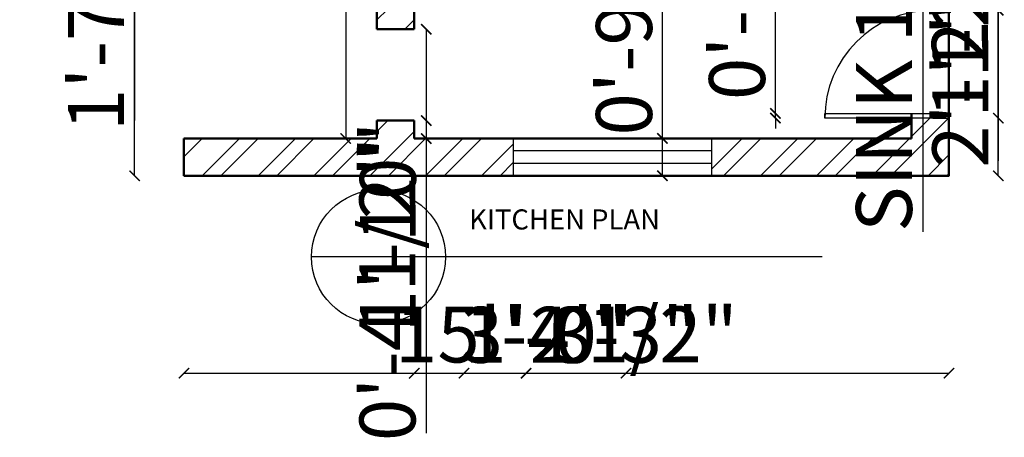
# Model space of a CAD drawing. Units: inches. Extents: x 1736 to 2023, y 1717 to 2014.
# Tile 1 of 3: x 1736 to 1974, y 1717 to 1818. Entities that reach past the tile are written whole.
import ezdxf

# ---------------------------------------------------------------- set-up
doc = ezdxf.new("R2010")
doc.units = ezdxf.units.IN
for name, color, linetype, lineweight in [('A-ANNO-DIMS', 2, 'Continuous', 18), ('A-ANNO-SYMB', 7, 'Continuous', 25), ('A-DOOR', 4, 'Continuous', 25), ('A-GLAZ', 4, 'Continuous', 25), ('A-WALL', 7, 'Continuous', 50), ('A-WALL-PATT', 8, 'Continuous', 13)]:
    doc.layers.add(name, color=color, linetype=linetype, lineweight=lineweight)
doc.styles.get("Standard").update_dxf_attribs({"font": 'arial.ttf'})
doc.dimstyles.new('ISO-25', dxfattribs={"dimtxt": 13.5, "dimasz": 2.5, "dimexe": 1.25, "dimexo": 0.625, "dimtad": 1, "dimdec": 0, "dimlunit": 4, "dimtxsty": 'Standard', "dimblk": 'ARCHTICK', "dimcen": 2.5, "dimse1": 1, "dimse2": 1, "dimclrd": 2, "dimclrt": 4, "dimadec": 0, "dimazin": 0, "dimtfac": 1, "dimtdec": 0, "dimtmove": 0, "dimatfit": 3, "dimfxl": 1, "dimarcsym": 0})

# ---------------------------------------------------------------- blocks, each defined once
blk = doc.blocks.new('*U4')
for p, q in [((0, 0), (0, -6)), ((40, 0), (40, -6))]:
    blk.add_line(p, q)
blk.add_lwpolyline([(0, 0), (0, 40), (1.75, 40), (1.75, 0)], close=True)
blk.add_arc((0, 0), 40, 0, 90)
blk = doc.blocks.new('_ArchTick')
at = {"color": 0, "linetype": 'ByBlock', "const_width": 0.15}
blk.add_lwpolyline([(-0.5, -0.5), (0.5, 0.5)], dxfattribs=at)
blk = doc.blocks.new('*D8')
at = {"layer": 'A-ANNO-DIMS', "color": 0, "lineweight": -2, "transparency": 16777216}
blk.add_line((1814.91, 1933.29), (1814.91, 1789.29), dxfattribs=at)
at = {"layer": 'Defpoints', "color": 0, "transparency": 16777216}
for p in [(1822.43, 1933.29), (1814.91, 1789.29), (1822.43, 1789.29)]:
    blk.add_point(p, dxfattribs=at)
at = {"layer": 'A-ANNO-DIMS', "color": 0, "lineweight": -2, "transparency": 16777216, "xscale": 2.5, "yscale": 2.5, "zscale": 2.5}
for p, rotation in [((1814.91, 1933.29), 90), ((1814.91, 1789.29), 270)]:
    blk.add_blockref('_ArchTick', p, dxfattribs=dict(at, rotation=rotation))
at = {"layer": 'A-ANNO-DIMS', "color": 0, "transparency": 16777216, "insert": (1807.51, 1861.29), "char_height": 13.5, "attachment_point": 5, "rotation": 90}
blk.add_mtext("12'", dxfattribs=at)
blk = doc.blocks.new('*D11')
at = {"layer": 'A-ANNO-DIMS', "color": 2, "lineweight": -2, "transparency": 16777216}
for p, q in [((1954.12, 1873.5), (1954.12, 1855.61)), ((1954.12, 1855.61), (1954.12, 1766.78))]:
    blk.add_line(p, q, dxfattribs=at)
at = {"layer": 'Defpoints', "color": 0, "transparency": 16777216}
for p in [(1951.43, 1873.5), (1951.43, 1855.61), (1954.12, 1855.61)]:
    blk.add_point(p, dxfattribs=at)
at = {"layer": 'A-ANNO-DIMS', "color": 2, "lineweight": -2, "transparency": 16777216, "xscale": 2.5, "yscale": 2.5, "zscale": 2.5}
for p, rotation in [((1954.12, 1873.5), 90), ((1954.12, 1855.61), 270)]:
    blk.add_blockref('_ArchTick', p, dxfattribs=dict(at, rotation=rotation))
at = {"layer": 'A-ANNO-DIMS', "color": 4, "transparency": 16777216, "insert": (1946.51, 1809.94), "char_height": 13.5, "attachment_point": 5, "rotation": 90}
blk.add_mtext('SINK 1\'-6"', dxfattribs=at)
blk = doc.blocks.new('*D13')
at = {"layer": 'A-ANNO-DIMS', "color": 2, "lineweight": -2, "transparency": 16777216}
blk.add_line((1775.89, 1732.64), (1960.43, 1732.64), dxfattribs=at)
at = {"layer": 'Defpoints', "color": 0, "transparency": 16777216}
for p in [(1775.89, 1780.29), (1960.43, 1780.29), (1960.43, 1732.64)]:
    blk.add_point(p, dxfattribs=at)
at = {"layer": 'A-ANNO-DIMS', "color": 2, "lineweight": -2, "transparency": 16777216, "xscale": 2.5, "yscale": 2.5, "zscale": 2.5, "rotation": 180}
blk.add_blockref('_ArchTick', (1775.89, 1732.64), dxfattribs=at)
at = {"layer": 'A-ANNO-DIMS', "color": 2, "lineweight": -2, "transparency": 16777216, "xscale": 2.5, "yscale": 2.5, "zscale": 2.5}
blk.add_blockref('_ArchTick', (1960.43, 1732.64), dxfattribs=at)
at = {"layer": 'A-ANNO-DIMS', "color": 4, "transparency": 16777216, "insert": (1868.16, 1740.24), "char_height": 13.5, "attachment_point": 5}
blk.add_mtext('15\'-4 1/2"', dxfattribs=at)
blk = doc.blocks.new('*D14')
at = {"layer": 'A-ANNO-DIMS', "color": 2, "lineweight": -2, "transparency": 16777216}
blk.add_line((1763.99, 1780.29), (1763.99, 1942.29), dxfattribs=at)
at = {"layer": 'Defpoints', "color": 0, "transparency": 16777216}
for p in [(1763.99, 1942.29), (1775.89, 1942.29), (1775.89, 1780.29)]:
    blk.add_point(p, dxfattribs=at)
at = {"layer": 'A-ANNO-DIMS', "color": 2, "lineweight": -2, "transparency": 16777216, "xscale": 2.5, "yscale": 2.5, "zscale": 2.5}
for p, rotation in [((1763.99, 1942.29), 90), ((1763.99, 1780.29), 270)]:
    blk.add_blockref('_ArchTick', p, dxfattribs=dict(at, rotation=rotation))
at = {"layer": 'A-ANNO-DIMS', "color": 4, "transparency": 16777216, "insert": (1756.47, 1861.29), "char_height": 13.5, "attachment_point": 5, "rotation": 90}
blk.add_mtext('13\'-6"', dxfattribs=at)
blk = doc.blocks.new('*D17')
at = {"layer": 'A-ANNO-DIMS', "color": 2, "lineweight": -2, "transparency": 16777216}
for p, q in [((1891.31, 1789.29), (1891.31, 1828.92)), ((1891.31, 1780.29), (1891.31, 1789.29))]:
    blk.add_line(p, q, dxfattribs=at)
at = {"layer": 'Defpoints', "color": 0, "transparency": 16777216}
for p in [(1891.31, 1789.29), (1903.21, 1789.29), (1903.21, 1780.29)]:
    blk.add_point(p, dxfattribs=at)
at = {"layer": 'A-ANNO-DIMS', "color": 2, "lineweight": -2, "transparency": 16777216, "xscale": 2.5, "yscale": 2.5, "zscale": 2.5}
for p, rotation in [((1891.31, 1789.29), 90), ((1891.31, 1780.29), 270)]:
    blk.add_blockref('_ArchTick', p, dxfattribs=dict(at, rotation=rotation))
at = {"layer": 'A-ANNO-DIMS', "color": 4, "transparency": 16777216, "insert": (1883.79, 1810.35), "char_height": 13.5, "attachment_point": 5, "rotation": 90}
blk.add_mtext('0\'-9"', dxfattribs=at)
blk = doc.blocks.new('*D18')
at = {"layer": 'A-ANNO-DIMS', "color": 2, "lineweight": -2, "transparency": 16777216}
for p, q in [((1822.43, 1827.58), (1831.43, 1827.58)), ((1831.43, 1827.58), (1871.07, 1827.58))]:
    blk.add_line(p, q, dxfattribs=at)
at = {"layer": 'Defpoints', "color": 0, "transparency": 16777216}
for p in [(1831.43, 1827.58), (1822.43, 1815.68), (1831.43, 1815.68)]:
    blk.add_point(p, dxfattribs=at)
at = {"layer": 'A-ANNO-DIMS', "color": 2, "lineweight": -2, "transparency": 16777216, "xscale": 2.5, "yscale": 2.5, "zscale": 2.5, "rotation": 180}
blk.add_blockref('_ArchTick', (1822.43, 1827.58), dxfattribs=at)
at = {"layer": 'A-ANNO-DIMS', "color": 2, "lineweight": -2, "transparency": 16777216, "xscale": 2.5, "yscale": 2.5, "zscale": 2.5}
blk.add_blockref('_ArchTick', (1831.43, 1827.58), dxfattribs=at)
at = {"layer": 'A-ANNO-DIMS', "color": 4, "transparency": 16777216, "insert": (1852.5, 1835.1), "char_height": 13.5, "attachment_point": 5}
blk.add_mtext('0\'-9"', dxfattribs=at)
blk = doc.blocks.new('*D20')
at = {"layer": 'A-ANNO-DIMS', "color": 2, "lineweight": -2, "transparency": 16777216}
for p, q in [((1834.33, 1815.68), (1834.33, 1793.62)), ((1834.33, 1793.62), (1834.33, 1744.77))]:
    blk.add_line(p, q, dxfattribs=at)
at = {"layer": 'Defpoints', "color": 0, "transparency": 16777216}
for p in [(1822.43, 1815.68), (1822.43, 1793.62), (1834.33, 1793.62)]:
    blk.add_point(p, dxfattribs=at)
at = {"layer": 'A-ANNO-DIMS', "color": 2, "lineweight": -2, "transparency": 16777216, "xscale": 2.5, "yscale": 2.5, "zscale": 2.5}
for p, rotation in [((1834.33, 1815.68), 90), ((1834.33, 1793.62), 270)]:
    blk.add_blockref('_ArchTick', p, dxfattribs=dict(at, rotation=rotation))
at = {"layer": 'A-ANNO-DIMS', "color": 4, "transparency": 16777216, "insert": (1826.82, 1767.94), "char_height": 13.5, "attachment_point": 5, "rotation": 90}
blk.add_mtext('1\'-10"', dxfattribs=at)
blk = doc.blocks.new('*D21')
at = {"layer": 'A-ANNO-DIMS', "color": 2, "lineweight": -2, "transparency": 16777216}
for p, q in [((1834.33, 1793.62), (1834.33, 1789.29)), ((1834.33, 1789.29), (1834.33, 1718.19))]:
    blk.add_line(p, q, dxfattribs=at)
at = {"layer": 'Defpoints', "color": 0, "transparency": 16777216}
for p in [(1822.43, 1793.62), (1822.43, 1789.29), (1834.33, 1789.29)]:
    blk.add_point(p, dxfattribs=at)
at = {"layer": 'A-ANNO-DIMS', "color": 2, "lineweight": -2, "transparency": 16777216, "xscale": 2.5, "yscale": 2.5, "zscale": 2.5}
for p, rotation in [((1834.33, 1793.62), 90), ((1834.33, 1789.29), 270)]:
    blk.add_blockref('_ArchTick', p, dxfattribs=dict(at, rotation=rotation))
at = {"layer": 'A-ANNO-DIMS', "color": 4, "transparency": 16777216, "insert": (1826.73, 1752.49), "char_height": 13.5, "attachment_point": 5, "rotation": 90}
blk.add_mtext('0\'-4 1/2"', dxfattribs=at)
blk = doc.blocks.new('*D22')
at = {"layer": 'A-ANNO-DIMS', "color": 2, "lineweight": -2, "transparency": 16777216}
for p, q in [((1831.43, 1954.19), (1855.31, 1954.19)), ((1855.31, 1954.19), (1895.17, 1954.19))]:
    blk.add_line(p, q, dxfattribs=at)
at = {"layer": 'Defpoints', "color": 0, "transparency": 16777216}
for p in [(1855.31, 1954.19), (1831.43, 1789.29), (1855.31, 1789.29)]:
    blk.add_point(p, dxfattribs=at)
at = {"layer": 'A-ANNO-DIMS', "color": 2, "lineweight": -2, "transparency": 16777216, "xscale": 2.5, "yscale": 2.5, "zscale": 2.5, "rotation": 180}
blk.add_blockref('_ArchTick', (1831.43, 1954.19), dxfattribs=at)
at = {"layer": 'A-ANNO-DIMS', "color": 2, "lineweight": -2, "transparency": 16777216, "xscale": 2.5, "yscale": 2.5, "zscale": 2.5}
blk.add_blockref('_ArchTick', (1855.31, 1954.19), dxfattribs=at)
at = {"layer": 'A-ANNO-DIMS', "color": 4, "transparency": 16777216, "insert": (1876.49, 1961.7), "char_height": 13.5, "attachment_point": 5}
blk.add_mtext('2\'-0"', dxfattribs=at)
blk = doc.blocks.new('*D23')
at = {"layer": 'A-ANNO-DIMS', "color": 2, "lineweight": -2, "transparency": 16777216}
blk.add_line((1855.31, 1954.19), (1903.21, 1954.19), dxfattribs=at)
at = {"layer": 'Defpoints', "color": 0, "transparency": 16777216}
for p in [(1903.21, 1954.19), (1855.31, 1789.29), (1903.21, 1789.29)]:
    blk.add_point(p, dxfattribs=at)
at = {"layer": 'A-ANNO-DIMS', "color": 2, "lineweight": -2, "transparency": 16777216, "xscale": 2.5, "yscale": 2.5, "zscale": 2.5, "rotation": 180}
blk.add_blockref('_ArchTick', (1855.31, 1954.19), dxfattribs=at)
at = {"layer": 'A-ANNO-DIMS', "color": 2, "lineweight": -2, "transparency": 16777216, "xscale": 2.5, "yscale": 2.5, "zscale": 2.5}
blk.add_blockref('_ArchTick', (1903.21, 1954.19), dxfattribs=at)
at = {"layer": 'A-ANNO-DIMS', "color": 4, "transparency": 16777216, "insert": (1879.26, 1961.7), "char_height": 13.5, "attachment_point": 5}
blk.add_mtext('4\'-0"', dxfattribs=at)
blk = doc.blocks.new('*D24')
at = {"layer": 'A-ANNO-DIMS', "color": 2, "lineweight": -2, "transparency": 16777216}
for p, q in [((1972.33, 1794.21), (1972.33, 1832.57)), ((1972.33, 1780.29), (1972.33, 1794.21))]:
    blk.add_line(p, q, dxfattribs=at)
at = {"layer": 'Defpoints', "color": 0, "transparency": 16777216}
for p in [(1960.43, 1794.21), (1972.33, 1794.21), (1960.43, 1780.29)]:
    blk.add_point(p, dxfattribs=at)
at = {"layer": 'A-ANNO-DIMS', "color": 2, "lineweight": -2, "transparency": 16777216, "xscale": 2.5, "yscale": 2.5, "zscale": 2.5}
for p, rotation in [((1972.33, 1794.21), 90), ((1972.33, 1780.29), 270)]:
    blk.add_blockref('_ArchTick', p, dxfattribs=dict(at, rotation=rotation))
at = {"layer": 'A-ANNO-DIMS', "color": 4, "transparency": 16777216, "insert": (1964.93, 1814.64), "char_height": 13.5, "attachment_point": 5, "rotation": 90}
blk.add_mtext('1\'-2"', dxfattribs=at)
blk = doc.blocks.new('*D25')
at = {"layer": 'A-ANNO-DIMS', "color": 2, "lineweight": -2, "transparency": 16777216}
for p, q in [((1972.33, 1820.25), (1972.33, 1860.12)), ((1972.33, 1794.21), (1972.33, 1820.25))]:
    blk.add_line(p, q, dxfattribs=at)
at = {"layer": 'Defpoints', "color": 0, "transparency": 16777216}
for p in [(1960.43, 1820.25), (1972.33, 1820.25), (1960.43, 1794.21)]:
    blk.add_point(p, dxfattribs=at)
at = {"layer": 'A-ANNO-DIMS', "color": 2, "lineweight": -2, "transparency": 16777216, "xscale": 2.5, "yscale": 2.5, "zscale": 2.5}
for p, rotation in [((1972.33, 1820.25), 90), ((1972.33, 1794.21), 270)]:
    blk.add_blockref('_ArchTick', p, dxfattribs=dict(at, rotation=rotation))
at = {"layer": 'A-ANNO-DIMS', "color": 4, "transparency": 16777216, "insert": (1964.93, 1841.44), "char_height": 13.5, "attachment_point": 5, "rotation": 90}
blk.add_mtext('2\'-2"', dxfattribs=at)
blk = doc.blocks.new('*D28')
at = {"layer": 'A-ANNO-DIMS', "color": 2, "lineweight": -2, "transparency": 16777216}
for p, q in [((1918.58, 1795.35), (1918.58, 1837.48)), ((1918.58, 1794.21), (1918.58, 1795.35)), ((1918.58, 1794.21), (1918.58, 1791.71))]:
    blk.add_line(p, q, dxfattribs=at)
at = {"layer": 'Defpoints', "color": 0, "transparency": 16777216}
for p in [(1918.58, 1795.35), (1930.48, 1795.35), (1930.48, 1794.21)]:
    blk.add_point(p, dxfattribs=at)
at = {"layer": 'A-ANNO-DIMS', "color": 2, "lineweight": -2, "transparency": 16777216, "xscale": 2.5, "yscale": 2.5, "zscale": 2.5}
for p, rotation in [((1918.58, 1795.35), 270), ((1918.58, 1794.21), 90)]:
    blk.add_blockref('_ArchTick', p, dxfattribs=dict(at, rotation=rotation))
at = {"layer": 'A-ANNO-DIMS', "color": 4, "transparency": 16777216, "insert": (1911.06, 1818.91), "char_height": 13.5, "attachment_point": 5, "rotation": 90}
blk.add_mtext('0\'-1"', dxfattribs=at)
blk = doc.blocks.new('*D32')
at = {"layer": 'A-ANNO-DIMS', "color": 2, "lineweight": -2, "transparency": 16777216}
for p, q in [((1831.43, 1732.64), (1843.43, 1732.64)), ((1843.43, 1732.64), (1881.8, 1732.64))]:
    blk.add_line(p, q, dxfattribs=at)
at = {"layer": 'Defpoints', "color": 0, "transparency": 16777216}
for p in [(1831.43, 1913.5), (1843.43, 1913.5), (1843.43, 1732.64)]:
    blk.add_point(p, dxfattribs=at)
at = {"layer": 'A-ANNO-DIMS', "color": 2, "lineweight": -2, "transparency": 16777216, "xscale": 2.5, "yscale": 2.5, "zscale": 2.5, "rotation": 180}
blk.add_blockref('_ArchTick', (1831.43, 1732.64), dxfattribs=at)
at = {"layer": 'A-ANNO-DIMS', "color": 2, "lineweight": -2, "transparency": 16777216, "xscale": 2.5, "yscale": 2.5, "zscale": 2.5}
blk.add_blockref('_ArchTick', (1843.43, 1732.64), dxfattribs=at)
at = {"layer": 'A-ANNO-DIMS', "color": 4, "transparency": 16777216, "insert": (1863.87, 1740.16), "char_height": 13.5, "attachment_point": 5}
blk.add_mtext('1\'-0"', dxfattribs=at)
blk = doc.blocks.new('*D33')
at = {"layer": 'A-ANNO-DIMS', "color": 2, "lineweight": -2, "transparency": 16777216}
for p, q in [((1831.43, 1732.64), (1858.43, 1732.64)), ((1858.43, 1732.64), (1898.3, 1732.64))]:
    blk.add_line(p, q, dxfattribs=at)
at = {"layer": 'Defpoints', "color": 0, "transparency": 16777216}
for p in [(1831.43, 1863.49), (1858.43, 1863.49), (1858.43, 1732.64)]:
    blk.add_point(p, dxfattribs=at)
at = {"layer": 'A-ANNO-DIMS', "color": 2, "lineweight": -2, "transparency": 16777216, "xscale": 2.5, "yscale": 2.5, "zscale": 2.5, "rotation": 180}
blk.add_blockref('_ArchTick', (1831.43, 1732.64), dxfattribs=at)
at = {"layer": 'A-ANNO-DIMS', "color": 2, "lineweight": -2, "transparency": 16777216, "xscale": 2.5, "yscale": 2.5, "zscale": 2.5}
blk.add_blockref('_ArchTick', (1858.43, 1732.64), dxfattribs=at)
at = {"layer": 'A-ANNO-DIMS', "color": 4, "transparency": 16777216, "insert": (1879.62, 1740.16), "char_height": 13.5, "attachment_point": 5}
blk.add_mtext('2\'-3"', dxfattribs=at)
blk = doc.blocks.new('*D42')
at = {"layer": 'A-ANNO-DIMS', "color": 2, "lineweight": -2, "transparency": 16777216}
for p, q in [((1763.99, 1883.21), (1763.99, 1863.49)), ((1763.99, 1863.49), (1763.99, 1793.67))]:
    blk.add_line(p, q, dxfattribs=at)
at = {"layer": 'Defpoints', "color": 0, "transparency": 16777216}
for p in [(1843.43, 1883.21), (1763.99, 1863.49), (1843.43, 1863.49)]:
    blk.add_point(p, dxfattribs=at)
at = {"layer": 'A-ANNO-DIMS', "color": 2, "lineweight": -2, "transparency": 16777216, "xscale": 2.5, "yscale": 2.5, "zscale": 2.5}
for p, rotation in [((1763.99, 1883.21), 90), ((1763.99, 1863.49), 270)]:
    blk.add_blockref('_ArchTick', p, dxfattribs=dict(at, rotation=rotation))
at = {"layer": 'A-ANNO-DIMS', "color": 4, "transparency": 16777216, "insert": (1756.39, 1827.33), "char_height": 13.5, "attachment_point": 5, "rotation": 90}
blk.add_mtext('1\'-7 1/2"', dxfattribs=at)
blk = doc.blocks.new('*D43')
at = {"layer": 'A-ANNO-DIMS', "color": 2, "lineweight": -2, "transparency": 16777216}
blk.add_line((1843.43, 1732.64), (1882.52, 1732.64), dxfattribs=at)
at = {"layer": 'Defpoints', "color": 0, "transparency": 16777216}
for p in [(1843.43, 1921.29), (1882.52, 1921.29), (1882.52, 1732.64)]:
    blk.add_point(p, dxfattribs=at)
at = {"layer": 'A-ANNO-DIMS', "color": 2, "lineweight": -2, "transparency": 16777216, "xscale": 2.5, "yscale": 2.5, "zscale": 2.5, "rotation": 180}
blk.add_blockref('_ArchTick', (1843.43, 1732.64), dxfattribs=at)
at = {"layer": 'A-ANNO-DIMS', "color": 2, "lineweight": -2, "transparency": 16777216, "xscale": 2.5, "yscale": 2.5, "zscale": 2.5}
blk.add_blockref('_ArchTick', (1882.52, 1732.64), dxfattribs=at)
at = {"layer": 'A-ANNO-DIMS', "color": 4, "transparency": 16777216, "insert": (1862.97, 1740.16), "char_height": 13.5, "attachment_point": 5}
blk.add_mtext('3\'-3"', dxfattribs=at)
blk = doc.blocks.new('*D47')
at = {"layer": 'A-ANNO-DIMS', "color": 2, "lineweight": -2, "transparency": 16777216}
for p, q in [((1972.33, 1878.88), (1972.33, 1848.88)), ((1972.33, 1848.88), (1972.33, 1809.01))]:
    blk.add_line(p, q, dxfattribs=at)
at = {"layer": 'Defpoints', "color": 0, "transparency": 16777216}
for p in [(1934.43, 1878.88), (1934.43, 1848.88), (1972.33, 1848.88)]:
    blk.add_point(p, dxfattribs=at)
at = {"layer": 'A-ANNO-DIMS', "color": 2, "lineweight": -2, "transparency": 16777216, "xscale": 2.5, "yscale": 2.5, "zscale": 2.5}
for p, rotation in [((1972.33, 1878.88), 90), ((1972.33, 1848.88), 270)]:
    blk.add_blockref('_ArchTick', p, dxfattribs=dict(at, rotation=rotation))
at = {"layer": 'A-ANNO-DIMS', "color": 4, "transparency": 16777216, "insert": (1964.82, 1827.7), "char_height": 13.5, "attachment_point": 5, "rotation": 90}
blk.add_mtext('2\'-6"', dxfattribs=at)
blk = doc.blocks.new('*D48')
at = {"layer": 'A-ANNO-DIMS', "color": 2, "lineweight": -2, "transparency": 16777216}
for p, q in [((1972.33, 1848.88), (1972.33, 1823.77)), ((1972.33, 1823.77), (1972.33, 1783.9))]:
    blk.add_line(p, q, dxfattribs=at)
at = {"layer": 'Defpoints', "color": 0, "transparency": 16777216}
for p in [(1934.43, 1848.88), (1934.43, 1823.77), (1972.33, 1823.77)]:
    blk.add_point(p, dxfattribs=at)
at = {"layer": 'A-ANNO-DIMS', "color": 2, "lineweight": -2, "transparency": 16777216, "xscale": 2.5, "yscale": 2.5, "zscale": 2.5}
for p, rotation in [((1972.33, 1848.88), 90), ((1972.33, 1823.77), 270)]:
    blk.add_blockref('_ArchTick', p, dxfattribs=dict(at, rotation=rotation))
at = {"layer": 'A-ANNO-DIMS', "color": 4, "transparency": 16777216, "insert": (1964.93, 1802.58), "char_height": 13.5, "attachment_point": 5, "rotation": 90}
blk.add_mtext('2\'-1"', dxfattribs=at)

msp = doc.modelspace()

# ---------------------------------------------------------------- hatches: boundary and pattern name
at = {"layer": 'A-WALL-PATT'}
h = msp.add_hatch(dxfattribs=at)
h.set_pattern_fill('ANSI32', color=256)
h.paths.add_polyline_path([(1831.43, 1933.29), (1884.52, 1933.29), (1884.52, 1933.93), (1910.52, 1933.93), (1910.52, 1933.29), (1951.43, 1933.29), (1951.43, 1911.39), (1960.43, 1911.39), (1960.43, 1942.29), (1822.43, 1942.29), (1775.89, 1942.29), (1775.89, 1933.29), (1822.43, 1933.29), (1822.43, 1815.68), (1831.43, 1815.68)])
h.paths.add_polyline_path([(1960.43, 1848.88), (1951.43, 1848.88), (1951.43, 1819.75, -0.049233), (1956.53, 1820.25), (1960.43, 1820.25)], flags=17)
h.paths.add_polyline_path([(1960.43, 1794.21), (1956.53, 1794.21), (1951.43, 1794.21), (1951.43, 1789.29), (1903.21, 1789.29), (1903.21, 1780.29), (1960.43, 1780.29)])
h.paths.add_polyline_path([(1855.31, 1789.29), (1831.43, 1789.29), (1831.43, 1793.62), (1822.43, 1793.62), (1822.43, 1789.29), (1775.89, 1789.29), (1775.89, 1780.29), (1822.43, 1780.29), (1855.31, 1780.29)])

# ---------------------------------------------------------------- linework, layer by layer
at = {"layer": 'A-ANNO-SYMB'}
for p, q in [((1822.81, 1760.71), (1806.64, 1760.71)), ((1929.86, 1760.71), (1822.81, 1760.71))]:
    msp.add_line(p, q, dxfattribs=at)
msp.add_circle((1822.81, 1760.71), 16.17, dxfattribs=at)
at = {"layer": 'A-GLAZ'}
for p, q in [((1855.31, 1789.29), (1855.31, 1780.29)), ((1903.21, 1789.29), (1855.31, 1789.29)), ((1903.21, 1780.29), (1903.21, 1789.29)), ((1903.21, 1786.29), (1855.31, 1786.29)), ((1903.21, 1783.29), (1855.31, 1783.29)), ((1855.31, 1780.29), (1903.21, 1780.29))]:
    msp.add_line(p, q, dxfattribs=at)
at = {"layer": 'A-WALL'}
for p, q in [((1831.43, 1815.68), (1831.43, 1933.29)), ((1831.43, 1815.68), (1822.43, 1815.68)), ((1831.43, 1793.62), (1822.43, 1793.62)), ((1831.43, 1789.29), (1831.43, 1793.62)), ((1951.43, 1795.35), (1951.43, 1789.29)), ((1775.89, 1780.29), (1775.89, 1789.29)), ((1775.89, 1789.29), (1822.43, 1789.29)), ((1951.43, 1789.29), (1831.43, 1789.29)), ((1775.89, 1780.29), (1822.43, 1780.29))]:
    msp.add_line(p, q, dxfattribs=at)
for points in [[(1822.43, 1942.29), (1960.43, 1942.29), (1960.43, 1780.29), (1822.43, 1780.29)], [(1822.43, 1815.68), (1822.43, 1933.29)], [(1822.43, 1789.29), (1822.43, 1793.62)]]:
    msp.add_lwpolyline(points, dxfattribs=at)

# ---------------------------------------------------------------- block references
at = {"layer": 'A-DOOR', "xscale": 0.651221867343762, "yscale": 0.651221867343762, "zscale": 0.651221867343762, "rotation": 90}
msp.add_blockref('*U4', (1956.53, 1794.21), dxfattribs=at)

# ---------------------------------------------------------------- texts
at = {"layer": 'A-ANNO-SYMB'}
msp.add_text('KITCHEN PLAN', height=4.8561, dxfattribs=at).set_placement((1844.69, 1767.33))

# ---------------------------------------------------------------- dimensions: what is measured, and where the dimension line sits
at = {"layer": 'A-ANNO-DIMS'}
for base, p1, p2, picture, middle in [((1855.31, 1954.19), (1831.43, 1789.29), (1855.31, 1789.29), '*D22', (1876.49, 1961.7)), ((1903.21, 1954.19), (1855.31, 1789.29), (1903.21, 1789.29), '*D23', (1879.26, 1961.7)), ((1882.52, 1732.64), (1843.43, 1921.29), (1882.52, 1921.29), '*D43', (1862.97, 1740.16)), ((1843.43, 1732.64), (1831.43, 1913.5), (1843.43, 1913.5), '*D32', (1863.87, 1740.16)), ((1858.43, 1732.64), (1831.43, 1863.49), (1858.43, 1863.49), '*D33', (1879.62, 1740.16)), ((1831.43, 1827.58), (1822.43, 1815.68), (1831.43, 1815.68), '*D18', (1852.5, 1835.1)), ((1960.43, 1732.64), (1775.89, 1780.29), (1960.43, 1780.29), '*D13', (1868.16, 1740.24))]:
    dim = msp.add_linear_dim(base=base, p1=p1, p2=p2, dimstyle='ISO-25', override={"dimdec": 1, "dimlfac": 1, "dimrnd": 0, "dimzin": 1, "dimdsep": 46, "dimlunit": 4, "dimfrac": 2}, dxfattribs=at)
    dim.commit()
    dim.dimension.update_dxf_attribs({"geometry": picture, "text_midpoint": middle})
for base, p1, p2, angle, override, picture, middle in [((1763.99, 1942.29), (1775.89, 1780.29), (1775.89, 1942.29), 90, {"dimdec": 1, "dimlfac": 1, "dimrnd": 0, "dimzin": 1, "dimdsep": 46, "dimlunit": 4, "dimfrac": 2}, '*D14', (1756.47, 1861.29)), ((1814.91, 1789.29), (1822.43, 1933.29), (1822.43, 1789.29), 90, {"dimclrd": 0, "dimclre": 0, "dimclrt": 0}, '*D8', (1807.51, 1861.29)), ((1763.99, 1863.49), (1843.43, 1883.21), (1843.43, 1863.49), 90, {"dimdec": 1, "dimlfac": 1, "dimrnd": 0, "dimzin": 1, "dimdsep": 46, "dimlunit": 4, "dimfrac": 2}, '*D42', (1756.39, 1827.33)), ((1972.33, 1848.88), (1934.43, 1878.88), (1934.43, 1848.88), 90, {"dimdec": 1, "dimlfac": 1, "dimrnd": 0, "dimzin": 1, "dimdsep": 46, "dimlunit": 4, "dimfrac": 2}, '*D47', (1964.82, 1827.7)), ((1972.33, 1820.25), (1960.43, 1794.21), (1960.43, 1820.25), 90, {"dimdec": 1, "dimlfac": 1, "dimrnd": 0, "dimzin": 1, "dimdsep": 46, "dimlunit": 4, "dimfrac": 2}, '*D25', (1964.93, 1841.44)), ((1972.33, 1823.77), (1934.43, 1848.88), (1934.43, 1823.77), 90, {"dimdec": 1, "dimlfac": 1, "dimrnd": 0, "dimzin": 1, "dimdsep": 46, "dimlunit": 4, "dimfrac": 2}, '*D48', (1964.93, 1802.58)), ((1918.58, 1795.35), (1930.48, 1794.21), (1930.48, 1795.35), 90, {"dimdec": 1, "dimlfac": 1, "dimrnd": 0, "dimzin": 1, "dimdsep": 46, "dimlunit": 4, "dimfrac": 2}, '*D28', (1911.06, 1818.91)), ((1972.33, 1794.21), (1960.43, 1780.29), (1960.43, 1794.21), 90, {"dimdec": 1, "dimlfac": 1, "dimrnd": 0, "dimzin": 1, "dimdsep": 46, "dimlunit": 4, "dimfrac": 2}, '*D24', (1964.93, 1814.64)), ((1891.31, 1789.29), (1903.21, 1780.29), (1903.21, 1789.29), 90, {"dimdec": 1, "dimlfac": 1, "dimrnd": 0, "dimzin": 1, "dimdsep": 46, "dimlunit": 4, "dimfrac": 2}, '*D17', (1883.79, 1810.35)), ((1834.33, 1793.62), (1822.43, 1815.68), (1822.43, 1793.62), 270, {"dimdec": 1, "dimlfac": 1, "dimrnd": 0, "dimzin": 1, "dimdsep": 46, "dimlunit": 4, "dimfrac": 2}, '*D20', (1826.82, 1767.94)), ((1834.33, 1789.29), (1822.43, 1793.62), (1822.43, 1789.29), 270, {"dimdec": 1, "dimlfac": 1, "dimrnd": 0, "dimzin": 1, "dimdsep": 46, "dimlunit": 4, "dimfrac": 2}, '*D21', (1826.73, 1752.49))]:
    dim = msp.add_linear_dim(base=base, p1=p1, p2=p2, angle=angle, dimstyle='ISO-25', override=override, dxfattribs=at)
    dim.commit()
    dim.dimension.update_dxf_attribs({"geometry": picture, "text_midpoint": middle})
dim = msp.add_linear_dim(base=(1954.12, 1855.61), p1=(1951.43, 1873.5), p2=(1951.43, 1855.61), angle=270, text='SINK <>', dimstyle='ISO-25', override={"dimdec": 1, "dimlfac": 1, "dimrnd": 0, "dimzin": 1, "dimdsep": 46, "dimlunit": 4, "dimfrac": 2}, dxfattribs=at)
dim.commit()
dim.dimension.update_dxf_attribs({"geometry": '*D11', "text_midpoint": (1946.51, 1809.94)})

doc.saveas('drawing.dxf')
